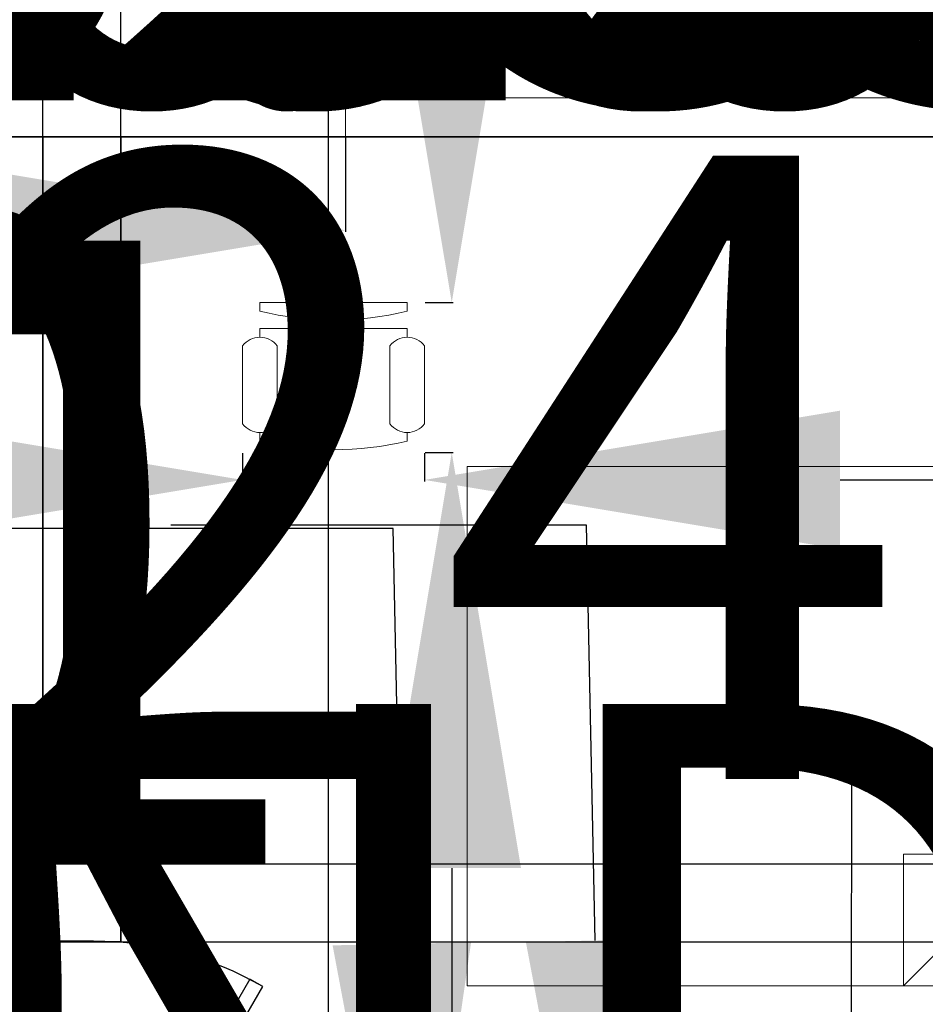
# Model space of a CAD drawing. Units: inches. Extents: x -307 to 2141, y -58 to 895.
# Tile 23 of 28: x 776 to 880, y 582 to 696. Entities that reach past the tile are written whole.
import ezdxf

# ---------------------------------------------------------------- set-up
doc = ezdxf.new("R2010")
doc.units = ezdxf.units.IN
doc.header["$MEASUREMENT"] = 0
for name, color, linetype, lineweight in [('A-ANNO-DIMS', 2, 'Continuous', 18), ('A-DOOR', 3, 'Continuous', 25), ('A-FURN', 8, 'Continuous', 18), ('A-GLAZ', 4, 'Continuous', 18), ('A-WALL', 7, 'Continuous', 35)]:
    doc.layers.add(name, color=color, linetype=linetype, lineweight=lineweight)
doc.styles.get("Standard").update_dxf_attribs({"font": 'arial.ttf'})
doc.dimstyles.get("Standard").update_dxf_attribs({"dimtxt": 72, "dimasz": 48, "dimexe": 0.18, "dimexo": 0.0625, "dimgap": 0.09, "dimtad": 0, "dimtih": 1, "dimtoh": 1, "dimdec": 0, "dimrnd": 48, "dimzin": 0, "dimdsep": 46, "dimlunit": 3, "dimtxsty": 'Standard', "dimcen": 0.09, "dimadec": 0, "dimazin": 0, "dimtfac": 1, "dimtdec": 0, "dimtofl": 0, "dimtmove": 0, "dimatfit": 3, "dimfxl": 1, "dimtolj": 1, "dimtzin": 0, "dimarcsym": 0})

# ---------------------------------------------------------------- blocks, each defined once
blk = doc.blocks.new('*U2')
for p, q in [((0, 0), (0, -6)), ((-40, 0), (-40, -6))]:
    blk.add_line(p, q)
blk.add_lwpolyline([(0, 0), (-34.64, 20), (-35.52, 18.48), (-0.87, -1.52)], close=True)
blk.add_arc((0, 0), 40, 150, 180)
blk = doc.blocks.new('Bed - Queen')
for p, q in [((0, -80.00003), (0, 0)), ((0, 0), (59.99999, 0)), ((59.99999, 0), (59.99999, -80.00003)), ((7.99999, -1.2), (28.79998, -1.2)), ((7.99999, -14.4), (7.99999, -1.2)), ((28.79998, -1.2), (28.79998, -14.4)), ((31.19999, -1.2), (51.99999, -1.2)), ((31.19999, -14.4), (31.19999, -1.2)), ((51.99999, -1.2), (51.99999, -16.4)), ((0, -14.4), (44.8, -14.4)), ((59.99999, -29.6), (44.8, -14.4)), ((44.8, -14.4), (44.8, -29.6)), ((44.8, -16.8), (0, -16.8)), ((51.99999, -16.4), (46.79936, -16.4)), ((44.8, -29.6), (59.99999, -29.6)), ((59.99999, -80.00003), (0, -80.00003))]:
    blk.add_line(p, q)
blk = doc.blocks.new('Chair - Desk')
for p, q in [((-8.5, 0), (-8.5, -1)), ((-8.5, 0), (8.5, 0)), ((8.5, 0), (8.5, -1)), ((-2, -3), (-2, -1.9355)), ((2, -1.9576), (2, -3)), ((-8.5, -3), (-8.5, -4)), ((-8.5, -3), (8.5, -3)), ((8.5, -3), (8.5, -4)), ((-10.5, -5), (-10.5, -14)), ((-6.5, -14), (-6.5, -5)), ((6.5, -5), (6.5, -14)), ((10.5, -14), (10.5, -5)), ((-8.5, -15), (-8.5, -16)), ((8.5, -15), (8.5, -16))]:
    blk.add_line(p, q)
for centre, radius, start, end in [((0, 34.625), 36.625, 256.5803, 283.4197), ((-8.5, -6.5), 2.5, 36.8699, 143.1301), ((8.5, -6.5), 2.5, 36.8699, 143.1301), ((-8.5, -12.5), 2.5, 216.8699, 323.1301), ((8.5, -12.5), 2.5, 216.8699, 323.1301), ((0, 19.625), 36.625, 256.5803, 283.4197)]:
    blk.add_arc(centre, radius, start, end)
blk = doc.blocks.new('WIN-72IN')
blk.add_line((72, 4.5), (0, 4.5))
blk.add_lwpolyline([(72, 0), (0, 0), (0, 9), (72, 9)], close=True)
blk = doc.blocks.new('*D30')
at = {"layer": 'A-ANNO-DIMS', "color": 0, "lineweight": -2, "transparency": 16777216}
for p, q in [((570.74, 532.83), (570.74, 580.83)), ((570.74, 580.83), (618.74, 580.83)), ((565.4, 484.83), (570.92, 484.83)), ((565.4, 448.83), (570.92, 448.83)), ((570.74, 400.83), (570.74, 352.83))]:
    blk.add_line(p, q, dxfattribs=at)
at = {"layer": 'A-ANNO-DIMS', "color": 0, "transparency": 16777216}
for points in [[(562.74, 532.83), (578.74, 532.83), (570.74, 484.83)], [(562.74, 400.83), (578.74, 400.83), (570.74, 448.83)]]:
    blk.add_solid(points, dxfattribs=at)
at = {"layer": 'Defpoints', "color": 0, "transparency": 16777216}
for p in [(565.34, 484.83), (570.74, 484.83), (565.34, 448.83)]:
    blk.add_point(p, dxfattribs=at)
at = {"layer": 'A-ANNO-DIMS', "color": 0, "transparency": 16777216, "insert": (1030.17, 580.83), "char_height": 72, "attachment_point": 5}
blk.add_mtext('\\A1;WINDOW 36 TYP.', dxfattribs=at)
blk = doc.blocks.new('*D32')
at = {"layer": 'A-ANNO-DIMS', "color": 0, "lineweight": -2, "transparency": 16777216}
for p, q in [((813.29, 682.28), (813.29, 671.36)), ((885.29, 682.28), (885.29, 671.36)), ((765.29, 671.54), (717.29, 671.54)), ((933.29, 671.54), (981.29, 671.54))]:
    blk.add_line(p, q, dxfattribs=at)
at = {"layer": 'A-ANNO-DIMS', "color": 0, "transparency": 16777216}
for points in [[(765.29, 679.54), (765.29, 663.54), (813.29, 671.54)], [(933.29, 679.54), (933.29, 663.54), (885.29, 671.54)]]:
    blk.add_solid(points, dxfattribs=at)
at = {"layer": 'Defpoints', "color": 0, "transparency": 16777216}
for p in [(813.29, 682.34), (885.29, 682.34), (885.29, 671.54)]:
    blk.add_point(p, dxfattribs=at)
at = {"layer": 'A-ANNO-DIMS', "color": 0, "transparency": 16777216, "insert": (1392.73, 671.54), "char_height": 72, "attachment_point": 5}
blk.add_mtext('\\A1;WINDOW 72 TYP.', dxfattribs=at)
blk = doc.blocks.new('*D36')
at = {"layer": 'A-ANNO-DIMS', "color": 0, "lineweight": -2, "transparency": 16777216}
for p, q in [((871.71, 562.4), (871.76, 610.4)), ((876.55, 514.4), (871.47, 514.4)), ((876.51, 481.35), (871.44, 481.36)), ((871.56, 433.36), (871.51, 385.36)), ((871.51, 385.36), (823.51, 385.36))]:
    blk.add_line(p, q, dxfattribs=at)
at = {"layer": 'A-ANNO-DIMS', "color": 0, "transparency": 16777216}
for points in [[(863.71, 562.41), (879.71, 562.4), (871.65, 514.4)], [(863.56, 433.37), (879.56, 433.35), (871.62, 481.36)]]:
    blk.add_solid(points, dxfattribs=at)
at = {"layer": 'Defpoints', "color": 0, "transparency": 16777216}
for p in [(876.61, 514.4), (871.62, 481.36), (876.57, 481.35)]:
    blk.add_point(p, dxfattribs=at)
at = {"layer": 'A-ANNO-DIMS', "color": 0, "transparency": 16777216, "insert": (548.95, 385.36), "char_height": 72, "attachment_point": 5}
blk.add_mtext('\\A1;WC 33 TYP.', dxfattribs=at)
blk = doc.blocks.new('*D37')
at = {"layer": 'A-ANNO-DIMS', "color": 0, "lineweight": -2, "transparency": 16777216}
for p, q in [((828.62, 519.41), (780.62, 519.46)), ((876.61, 514.46), (876.62, 519.54)), ((897.61, 514.44), (897.62, 519.51)), ((945.62, 519.28), (993.62, 519.22))]:
    blk.add_line(p, q, dxfattribs=at)
at = {"layer": 'A-ANNO-DIMS', "color": 0, "transparency": 16777216}
for points in [[(828.63, 527.41), (828.61, 511.41), (876.62, 519.36)], [(945.63, 527.28), (945.61, 511.28), (897.62, 519.33)]]:
    blk.add_solid(points, dxfattribs=at)
at = {"layer": 'Defpoints', "color": 0, "transparency": 16777216}
for p in [(876.62, 519.36), (876.61, 514.4), (897.61, 514.38)]:
    blk.add_point(p, dxfattribs=at)
at = {"layer": 'A-ANNO-DIMS', "color": 0, "transparency": 16777216, "insert": (604.68, 519.46), "char_height": 72, "attachment_point": 5}
blk.add_mtext('\\A1;21 TYP.', dxfattribs=at)
blk = doc.blocks.new('*D42')
at = {"layer": 'A-ANNO-DIMS', "color": 0, "lineweight": -2, "transparency": 16777216}
for p, q in [((880.26, 543.86), (928.25, 544.87)), ((822.3, 541.2), (822.27, 542.82)), ((832.3, 541.41), (832.27, 543.03)), ((774.28, 541.63), (726.29, 540.62))]:
    blk.add_line(p, q, dxfattribs=at)
at = {"layer": 'A-ANNO-DIMS', "color": 0, "transparency": 16777216}
for points in [[(880.09, 551.86), (880.43, 535.86), (832.27, 542.85)], [(774.11, 549.63), (774.45, 533.63), (822.27, 542.64)]]:
    blk.add_solid(points, dxfattribs=at)
at = {"layer": 'Defpoints', "color": 0, "transparency": 16777216}
for p in [(832.27, 542.85), (822.3, 541.14), (832.3, 541.35)]:
    blk.add_point(p, dxfattribs=at)
at = {"layer": 'A-ANNO-DIMS', "color": 0, "transparency": 16777216, "insert": (1192.89, 544.87), "char_height": 72, "attachment_point": 5}
blk.add_mtext('\\A1;FAUCET 10', dxfattribs=at)
blk = doc.blocks.new('*D43')
at = {"layer": 'A-ANNO-DIMS', "color": 0, "lineweight": -2, "transparency": 16777216}
for p, q in [((818.79, 637.09), (770.79, 637.09)), ((819.79, 589.1), (818.79, 637.09)), ((822.24, 541.14), (820.62, 541.1)), ((822.38, 534.64), (820.76, 534.61)), ((821.95, 486.62), (822.96, 438.63))]:
    blk.add_line(p, q, dxfattribs=at)
at = {"layer": 'A-ANNO-DIMS', "color": 0, "transparency": 16777216}
for points in [[(827.79, 589.27), (811.8, 588.93), (820.8, 541.11)], [(829.95, 486.79), (813.95, 486.45), (820.94, 534.61)]]:
    blk.add_solid(points, dxfattribs=at)
at = {"layer": 'Defpoints', "color": 0, "transparency": 16777216}
for p in [(820.8, 541.11), (822.3, 541.14), (822.44, 534.64)]:
    blk.add_point(p, dxfattribs=at)
at = {"layer": 'A-ANNO-DIMS', "color": 0, "transparency": 16777216, "insert": (747.39, 637.09), "char_height": 72, "attachment_point": 5}
blk.add_mtext('\\A1;7', dxfattribs=at)
blk = doc.blocks.new('*D44')
at = {"layer": 'A-ANNO-DIMS', "color": 0, "lineweight": -2, "transparency": 16777216}
for p, q in [((839.87, 521.22), (839.95, 517.42)), ((815.33, 520.71), (815.41, 516.91)), ((887.94, 518.61), (935.93, 519.62)), ((767.41, 516.08), (719.42, 515.07))]:
    blk.add_line(p, q, dxfattribs=at)
at = {"layer": 'A-ANNO-DIMS', "color": 0, "transparency": 16777216}
for points in [[(887.77, 526.61), (888.11, 510.61), (839.95, 517.6)], [(767.25, 524.08), (767.58, 508.08), (815.4, 517.09)]]:
    blk.add_solid(points, dxfattribs=at)
at = {"layer": 'Defpoints', "color": 0, "transparency": 16777216}
for p in [(839.87, 521.29), (815.33, 520.77), (839.95, 517.6)]:
    blk.add_point(p, dxfattribs=at)
at = {"layer": 'A-ANNO-DIMS', "color": 0, "transparency": 16777216, "insert": (1151.16, 519.62), "char_height": 72, "attachment_point": 5}
blk.add_mtext('\\A1;BASIN 25', dxfattribs=at)
blk = doc.blocks.new('*D45')
at = {"layer": 'A-ANNO-DIMS', "color": 0, "lineweight": -2, "transparency": 16777216}
for p, q in [((841.11, 637.47), (793.11, 637.47)), ((842.12, 589.48), (841.11, 637.47)), ((839.51, 541.42), (843.31, 541.5)), ((839.93, 521.29), (843.73, 521.37)), ((844.56, 473.37), (845.57, 425.38))]:
    blk.add_line(p, q, dxfattribs=at)
at = {"layer": 'A-ANNO-DIMS', "color": 0, "transparency": 16777216}
for points in [[(850.12, 589.65), (834.12, 589.32), (843.13, 541.49)], [(852.56, 473.54), (836.56, 473.21), (843.55, 521.36)]]:
    blk.add_solid(points, dxfattribs=at)
at = {"layer": 'Defpoints', "color": 0, "transparency": 16777216}
for p in [(843.13, 541.49), (839.45, 541.42), (839.87, 521.29)]:
    blk.add_point(p, dxfattribs=at)
at = {"layer": 'A-ANNO-DIMS', "color": 0, "transparency": 16777216, "insert": (740.96, 637.47), "char_height": 72, "attachment_point": 5}
blk.add_mtext('\\A1;20', dxfattribs=at)
blk = doc.blocks.new('*D46')
at = {"layer": 'A-ANNO-DIMS', "color": 0, "lineweight": -2, "transparency": 16777216}
for p, q in [((801.41, 645.78), (801.41, 642.52)), ((822.41, 645.78), (822.41, 642.52)), ((753.41, 642.7), (705.41, 642.7)), ((870.41, 642.7), (918.41, 642.7))]:
    blk.add_line(p, q, dxfattribs=at)
at = {"layer": 'A-ANNO-DIMS', "color": 0, "transparency": 16777216}
for points in [[(753.41, 650.7), (753.41, 634.7), (801.41, 642.7)], [(870.41, 650.7), (870.41, 634.7), (822.41, 642.7)]]:
    blk.add_solid(points, dxfattribs=at)
at = {"layer": 'Defpoints', "color": 0, "transparency": 16777216}
for p in [(801.41, 645.85), (822.41, 645.85), (822.41, 642.7)]:
    blk.add_point(p, dxfattribs=at)
at = {"layer": 'A-ANNO-DIMS', "color": 0, "transparency": 16777216, "insert": (1282.7, 642.7), "char_height": 72, "attachment_point": 5}
blk.add_mtext('\\A1;DESK CHAIR 21', dxfattribs=at)
blk = doc.blocks.new('*D47')
at = {"layer": 'A-ANNO-DIMS', "color": 0, "lineweight": -2, "transparency": 16777216}
for p, q in [((825.56, 711.18), (825.56, 759.18)), ((825.56, 759.18), (873.56, 759.18)), ((822.48, 663.18), (825.74, 663.18)), ((822.48, 645.85), (825.74, 645.85)), ((825.56, 597.85), (825.56, 549.85))]:
    blk.add_line(p, q, dxfattribs=at)
at = {"layer": 'A-ANNO-DIMS', "color": 0, "transparency": 16777216}
for points in [[(817.56, 711.18), (833.56, 711.18), (825.56, 663.18)], [(817.56, 597.85), (833.56, 597.85), (825.56, 645.85)]]:
    blk.add_solid(points, dxfattribs=at)
at = {"layer": 'Defpoints', "color": 0, "transparency": 16777216}
for p in [(822.41, 663.18), (825.56, 663.18), (822.41, 645.85)]:
    blk.add_point(p, dxfattribs=at)
at = {"layer": 'A-ANNO-DIMS', "color": 0, "transparency": 16777216, "insert": (921.83, 759.18), "char_height": 72, "attachment_point": 5}
blk.add_mtext('\\A1;17', dxfattribs=at)
blk = doc.blocks.new('*D52')
at = {"layer": 'A-ANNO-DIMS', "color": 0, "lineweight": -2, "transparency": 16777216}
for p, q in [((660.21, 554.25), (660.21, 602.25)), ((673.8, 506.25), (660.03, 506.25)), ((673.8, 415.25), (660.03, 415.25)), ((660.21, 367.25), (660.21, 319.25))]:
    blk.add_line(p, q, dxfattribs=at)
at = {"layer": 'A-ANNO-DIMS', "color": 0, "transparency": 16777216}
for points in [[(652.21, 554.25), (668.21, 554.25), (660.21, 506.25)], [(652.21, 367.25), (668.21, 367.25), (660.21, 415.25)]]:
    blk.add_solid(points, dxfattribs=at)
at = {"layer": 'Defpoints', "color": 0, "transparency": 16777216}
for p in [(673.86, 506.25), (660.21, 415.25), (673.86, 415.25)]:
    blk.add_point(p, dxfattribs=at)
at = {"layer": 'A-ANNO-DIMS', "color": 0, "transparency": 16777216, "insert": (660.21, 460.75), "char_height": 72, "attachment_point": 5}
blk.add_mtext('\\A1;DINING SET 91', dxfattribs=at)
blk = doc.blocks.new('*D56')
at = {"layer": 'A-ANNO-DIMS', "color": 0, "lineweight": -2, "transparency": 16777216}
for p, q in [((679.73, 723.21), (679.73, 771.21)), ((679.73, 771.21), (727.73, 771.21)), ((675.74, 675.21), (679.91, 675.21)), ((675.74, 648.21), (679.91, 648.21)), ((679.73, 600.21), (679.73, 552.21))]:
    blk.add_line(p, q, dxfattribs=at)
at = {"layer": 'A-ANNO-DIMS', "color": 0, "transparency": 16777216}
for points in [[(671.73, 723.21), (687.73, 723.21), (679.73, 675.21)], [(671.73, 600.21), (687.73, 600.21), (679.73, 648.21)]]:
    blk.add_solid(points, dxfattribs=at)
at = {"layer": 'Defpoints', "color": 0, "transparency": 16777216}
for p in [(675.68, 675.21), (679.73, 675.21), (675.68, 648.21)]:
    blk.add_point(p, dxfattribs=at)
at = {"layer": 'A-ANNO-DIMS', "color": 0, "transparency": 16777216, "insert": (1006.66, 771.21), "char_height": 72, "attachment_point": 5}
blk.add_mtext('\\A1;ROCKER 27', dxfattribs=at)
blk = doc.blocks.new('*D57')
at = {"layer": 'A-ANNO-DIMS', "color": 0, "lineweight": -2, "transparency": 16777216}
for p, q in [((651.25, 648.15), (651.25, 643.98)), ((675.68, 648.15), (675.68, 643.98)), ((603.25, 644.16), (555.25, 644.16)), ((723.68, 644.16), (771.68, 644.16))]:
    blk.add_line(p, q, dxfattribs=at)
at = {"layer": 'A-ANNO-DIMS', "color": 0, "transparency": 16777216}
for points in [[(603.25, 652.16), (603.25, 636.16), (651.25, 644.16)], [(723.68, 652.16), (723.68, 636.16), (675.68, 644.16)]]:
    blk.add_solid(points, dxfattribs=at)
at = {"layer": 'Defpoints', "color": 0, "transparency": 16777216}
for p in [(651.25, 648.21), (675.68, 648.21), (675.68, 644.16)]:
    blk.add_point(p, dxfattribs=at)
at = {"layer": 'A-ANNO-DIMS', "color": 0, "transparency": 16777216, "insert": (823.81, 644.16), "char_height": 72, "attachment_point": 5}
blk.add_mtext('\\A1;24', dxfattribs=at)
blk = doc.blocks.new('*D62')
at = {"layer": 'A-ANNO-DIMS', "color": 0, "lineweight": -2, "transparency": 16777216}
for p, q in [((556.34, 691.4), (556.34, 722.72)), ((604.34, 722.54), (656.85, 722.54)), ((868.34, 722.54), (815.82, 722.54)), ((916.34, 490.97), (916.34, 722.72))]:
    blk.add_line(p, q, dxfattribs=at)
at = {"layer": 'A-ANNO-DIMS', "color": 0, "transparency": 16777216}
for points in [[(604.34, 730.54), (604.34, 714.54), (556.34, 722.54)], [(868.34, 730.54), (868.34, 714.54), (916.34, 722.54)]]:
    blk.add_solid(points, dxfattribs=at)
at = {"layer": 'Defpoints', "color": 0, "transparency": 16777216}
for p in [(916.34, 722.54), (556.34, 691.34), (916.34, 490.9)]:
    blk.add_point(p, dxfattribs=at)
at = {"layer": 'A-ANNO-DIMS', "color": 0, "transparency": 16777216, "insert": (736.34, 722.54), "char_height": 72, "attachment_point": 5}
blk.add_mtext('\\A1;360', dxfattribs=at)
blk = doc.blocks.new('*D63')
at = {"layer": 'A-ANNO-DIMS', "color": 0, "lineweight": -2, "transparency": 16777216}
for p, q in [((916.4, 691.34), (947.72, 691.34)), ((947.54, 643.34), (947.54, 416.19)), ((947.54, 115.34), (947.54, 342.49)), ((704.68, 67.34), (947.72, 67.34))]:
    blk.add_line(p, q, dxfattribs=at)
at = {"layer": 'A-ANNO-DIMS', "color": 0, "transparency": 16777216}
for points in [[(939.54, 643.34), (955.54, 643.34), (947.54, 691.34)], [(939.54, 115.34), (955.54, 115.34), (947.54, 67.34)]]:
    blk.add_solid(points, dxfattribs=at)
at = {"layer": 'Defpoints', "color": 0, "transparency": 16777216}
for p in [(916.34, 691.34), (704.62, 67.34), (947.54, 67.34)]:
    blk.add_point(p, dxfattribs=at)
at = {"layer": 'A-ANNO-DIMS', "color": 0, "transparency": 16777216, "insert": (947.54, 379.34), "char_height": 72, "attachment_point": 5}
blk.add_mtext('\\A1;624', dxfattribs=at)
blk = doc.blocks.new('*D68')
at = {"layer": 'A-ANNO-DIMS', "color": 0, "lineweight": -2, "transparency": 16777216}
for p, q in [((525.13, 586.34), (525.13, 634.34)), ((525.13, 634.34), (573.13, 634.34)), ((565.27, 538.34), (524.95, 538.34)), ((556.27, 484.83), (524.95, 484.83)), ((525.13, 436.83), (525.13, 388.83))]:
    blk.add_line(p, q, dxfattribs=at)
at = {"layer": 'A-ANNO-DIMS', "color": 0, "transparency": 16777216}
for points in [[(517.13, 586.34), (533.13, 586.34), (525.13, 538.34)], [(517.13, 436.83), (533.13, 436.83), (525.13, 484.83)]]:
    blk.add_solid(points, dxfattribs=at)
at = {"layer": 'Defpoints', "color": 0, "transparency": 16777216}
for p in [(525.13, 538.34), (565.34, 538.34), (556.34, 484.83)]:
    blk.add_point(p, dxfattribs=at)
at = {"layer": 'A-ANNO-DIMS', "color": 0, "transparency": 16777216, "insert": (687.75, 634.34), "char_height": 72, "attachment_point": 5}
blk.add_mtext('\\A1;53.51', dxfattribs=at)
blk = doc.blocks.new('*D75')
at = {"layer": 'A-ANNO-DIMS', "color": 0, "lineweight": -2, "transparency": 16777216}
for p, q in [((565.34, 682.4), (565.34, 722.72)), ((613.34, 722.54), (637.34, 722.54)), ((685.34, 682.4), (685.34, 722.72)), ((685.34, 722.54), (733.34, 722.54))]:
    blk.add_line(p, q, dxfattribs=at)
at = {"layer": 'A-ANNO-DIMS', "color": 0, "transparency": 16777216}
for points in [[(613.34, 730.54), (613.34, 714.54), (565.34, 722.54)], [(637.34, 730.54), (637.34, 714.54), (685.34, 722.54)]]:
    blk.add_solid(points, dxfattribs=at)
at = {"layer": 'Defpoints', "color": 0, "transparency": 16777216}
for p in [(685.34, 722.54), (565.34, 682.34), (685.34, 682.34)]:
    blk.add_point(p, dxfattribs=at)
at = {"layer": 'A-ANNO-DIMS', "color": 0, "transparency": 16777216, "insert": (809.45, 722.54), "char_height": 72, "attachment_point": 5}
blk.add_mtext('\\A1;120', dxfattribs=at)
blk = doc.blocks.new('*D76')
at = {"layer": 'A-ANNO-DIMS', "color": 0, "lineweight": -2, "transparency": 16777216}
for p, q in [((646.34, 722.54), (598.34, 722.54)), ((694.34, 682.4), (694.34, 722.72)), ((778.34, 682.4), (778.34, 722.72)), ((826.34, 722.54), (874.34, 722.54))]:
    blk.add_line(p, q, dxfattribs=at)
at = {"layer": 'A-ANNO-DIMS', "color": 0, "transparency": 16777216}
for points in [[(646.34, 730.54), (646.34, 714.54), (694.34, 722.54)], [(826.34, 730.54), (826.34, 714.54), (778.34, 722.54)]]:
    blk.add_solid(points, dxfattribs=at)
at = {"layer": 'Defpoints', "color": 0, "transparency": 16777216}
for p in [(778.34, 722.54), (694.34, 682.34), (778.34, 682.34)]:
    blk.add_point(p, dxfattribs=at)
at = {"layer": 'A-ANNO-DIMS', "color": 0, "transparency": 16777216, "insert": (925.9, 722.54), "char_height": 72, "attachment_point": 5}
blk.add_mtext('\\A1;84', dxfattribs=at)
blk = doc.blocks.new('*D77')
at = {"layer": 'A-ANNO-DIMS', "color": 0, "lineweight": -2, "transparency": 16777216}
for p, q in [((787.34, 682.4), (787.34, 722.72)), ((835.34, 722.54), (859.34, 722.54)), ((907.34, 682.4), (907.34, 722.72)), ((907.34, 722.54), (955.34, 722.54))]:
    blk.add_line(p, q, dxfattribs=at)
at = {"layer": 'A-ANNO-DIMS', "color": 0, "transparency": 16777216}
for points in [[(835.34, 730.54), (835.34, 714.54), (787.34, 722.54)], [(859.34, 730.54), (859.34, 714.54), (907.34, 722.54)]]:
    blk.add_solid(points, dxfattribs=at)
at = {"layer": 'Defpoints', "color": 0, "transparency": 16777216}
for p in [(907.34, 722.54), (787.34, 682.34), (907.34, 682.34)]:
    blk.add_point(p, dxfattribs=at)
at = {"layer": 'A-ANNO-DIMS', "color": 0, "transparency": 16777216, "insert": (1031.45, 722.54), "char_height": 72, "attachment_point": 5}
blk.add_mtext('\\A1;120', dxfattribs=at)
blk = doc.blocks.new('*D78')
at = {"layer": 'A-ANNO-DIMS', "color": 0, "lineweight": -2, "transparency": 16777216}
for p, q in [((947.53984, 730.340828), (947.53984, 778.340828)), ((778.39834, 682.340828), (947.71984, 682.340828)), ((730.39834, 598.340828), (947.71984, 598.340828)), ((947.53984, 550.340828), (947.53984, 502.340828))]:
    blk.add_line(p, q, dxfattribs=at)
at = {"layer": 'A-ANNO-DIMS', "color": 0, "transparency": 16777216}
for points in [[(939.53984, 730.340828), (955.53984, 730.340828), (947.53984, 682.340828)], [(939.53984, 550.340828), (955.53984, 550.340828), (947.53984, 598.340828)]]:
    blk.add_solid(points, dxfattribs=at)
at = {"layer": 'Defpoints', "color": 0, "transparency": 16777216}
for p in [(778.33584, 682.340828), (947.53984, 682.340828), (730.33584, 598.340828)]:
    blk.add_point(p, dxfattribs=at)
at = {"layer": 'A-ANNO-DIMS', "color": 0, "transparency": 16777216, "insert": (947.53984, 640.340828), "char_height": 72, "attachment_point": 5}
blk.add_mtext('\\A1;84', dxfattribs=at)
blk = doc.blocks.new('*D80')
at = {"layer": 'A-ANNO-DIMS', "color": 0, "lineweight": -2, "transparency": 16777216}
for p, q in [((763.34, 722.54), (715.34, 722.54)), ((811.34, 517.4), (811.34, 722.72)), ((907.34, 541.4), (907.34, 722.72)), ((955.34, 722.54), (1003.34, 722.54))]:
    blk.add_line(p, q, dxfattribs=at)
at = {"layer": 'A-ANNO-DIMS', "color": 0, "transparency": 16777216}
for points in [[(763.34, 730.54), (763.34, 714.54), (811.34, 722.54)], [(955.34, 730.54), (955.34, 714.54), (907.34, 722.54)]]:
    blk.add_solid(points, dxfattribs=at)
at = {"layer": 'Defpoints', "color": 0, "transparency": 16777216}
for p in [(907.34, 722.54), (907.34, 541.34), (811.34, 517.34)]:
    blk.add_point(p, dxfattribs=at)
at = {"layer": 'A-ANNO-DIMS', "color": 0, "transparency": 16777216, "insert": (1054.97, 722.54), "char_height": 72, "attachment_point": 5}
blk.add_mtext('\\A1;96', dxfattribs=at)
blk = doc.blocks.new('*D82')
at = {"layer": 'A-ANNO-DIMS', "color": 0, "lineweight": -2, "transparency": 16777216}
for p, q in [((525.13, 565.34), (525.13, 613.34)), ((525.13, 613.34), (573.13, 613.34)), ((802.27, 517.34), (524.95, 517.34)), ((802.27, 481.34), (524.95, 481.34)), ((525.13, 433.34), (525.13, 385.34))]:
    blk.add_line(p, q, dxfattribs=at)
at = {"layer": 'A-ANNO-DIMS', "color": 0, "transparency": 16777216}
for points in [[(517.13, 565.34), (533.13, 565.34), (525.13, 517.34)], [(517.13, 433.34), (533.13, 433.34), (525.13, 481.34)]]:
    blk.add_solid(points, dxfattribs=at)
at = {"layer": 'Defpoints', "color": 0, "transparency": 16777216}
for p in [(525.13, 517.34), (802.34, 517.34), (802.34, 481.34)]:
    blk.add_point(p, dxfattribs=at)
at = {"layer": 'A-ANNO-DIMS', "color": 0, "transparency": 16777216, "insert": (624.74, 613.34), "char_height": 72, "attachment_point": 5}
blk.add_mtext('\\A1;36', dxfattribs=at)
blk = doc.blocks.new('*D83')
at = {"layer": 'A-ANNO-DIMS', "color": 0, "lineweight": -2, "transparency": 16777216}
for p, q in [((947.54, 538.9), (947.54, 586.9)), ((916.4, 490.9), (947.72, 490.9)), ((907.4, 481.34), (947.72, 481.34)), ((947.54, 433.34), (947.54, 385.34)), ((947.54, 385.34), (899.54, 385.34))]:
    blk.add_line(p, q, dxfattribs=at)
at = {"layer": 'A-ANNO-DIMS', "color": 0, "transparency": 16777216}
for points in [[(939.54, 538.9), (955.54, 538.9), (947.54, 490.9)], [(939.54, 433.34), (955.54, 433.34), (947.54, 481.34)]]:
    blk.add_solid(points, dxfattribs=at)
at = {"layer": 'Defpoints', "color": 0, "transparency": 16777216}
for p in [(916.34, 490.9), (907.34, 481.34), (947.54, 481.34)]:
    blk.add_point(p, dxfattribs=at)
at = {"layer": 'A-ANNO-DIMS', "color": 0, "transparency": 16777216, "insert": (777.97, 385.34), "char_height": 72, "attachment_point": 5}
blk.add_mtext('\\A1;9.563', dxfattribs=at)
blk = doc.blocks.new('*D88')
at = {"layer": 'A-ANNO-DIMS', "color": 0, "lineweight": -2, "transparency": 16777216}
for p, q in [((517.33584, 722.544828), (469.33584, 722.544828)), ((565.33584, 295.403328), (565.33584, 722.724828)), ((754.33584, 271.403328), (754.33584, 722.724828)), ((802.33584, 722.544828), (850.33584, 722.544828))]:
    blk.add_line(p, q, dxfattribs=at)
at = {"layer": 'A-ANNO-DIMS', "color": 0, "transparency": 16777216}
for points in [[(517.33584, 730.544828), (517.33584, 714.544828), (565.33584, 722.544828)], [(802.33584, 730.544828), (802.33584, 714.544828), (754.33584, 722.544828)]]:
    blk.add_solid(points, dxfattribs=at)
at = {"layer": 'Defpoints', "color": 0, "transparency": 16777216}
for p in [(754.33584, 722.544828), (565.33584, 295.340828), (754.33584, 271.340828)]:
    blk.add_point(p, dxfattribs=at)
at = {"layer": 'A-ANNO-DIMS', "color": 0, "transparency": 16777216, "insert": (659.83584, 722.544828), "char_height": 72, "attachment_point": 5}
blk.add_mtext('\\A1;189', dxfattribs=at)
blk = doc.blocks.new('*D94')
at = {"layer": 'A-ANNO-DIMS', "color": 0, "lineweight": -2, "transparency": 16777216}
for p, q in [((517.34, 722.54), (469.34, 722.54)), ((565.34, 529.4), (565.34, 722.72)), ((629.84, 529.4), (629.84, 722.72)), ((677.84, 722.54), (725.84, 722.54))]:
    blk.add_line(p, q, dxfattribs=at)
at = {"layer": 'A-ANNO-DIMS', "color": 0, "transparency": 16777216}
for points in [[(517.34, 730.54), (517.34, 714.54), (565.34, 722.54)], [(677.84, 730.54), (677.84, 714.54), (629.84, 722.54)]]:
    blk.add_solid(points, dxfattribs=at)
at = {"layer": 'Defpoints', "color": 0, "transparency": 16777216}
for p in [(629.84, 722.54), (565.34, 529.34), (629.84, 529.34)]:
    blk.add_point(p, dxfattribs=at)
at = {"layer": 'A-ANNO-DIMS', "color": 0, "transparency": 16777216, "insert": (819.9, 722.54), "char_height": 72, "attachment_point": 5}
blk.add_mtext('\\A1;64.5', dxfattribs=at)
blk = doc.blocks.new('*D95')
at = {"layer": 'A-ANNO-DIMS', "color": 0, "lineweight": -2, "transparency": 16777216}
for p, q in [((947.54, 577.34), (947.54, 625.34)), ((947.54, 625.34), (995.54, 625.34)), ((629.9, 529.34), (947.72, 529.34)), ((629.9, 502.66), (947.72, 502.66)), ((947.54, 454.66), (947.54, 406.66))]:
    blk.add_line(p, q, dxfattribs=at)
at = {"layer": 'A-ANNO-DIMS', "color": 0, "transparency": 16777216}
for points in [[(939.54, 577.34), (955.54, 577.34), (947.54, 529.34)], [(939.54, 454.66), (955.54, 454.66), (947.54, 502.66)]]:
    blk.add_solid(points, dxfattribs=at)
at = {"layer": 'Defpoints', "color": 0, "transparency": 16777216}
for p in [(629.84, 529.34), (947.54, 529.34), (629.84, 502.66)]:
    blk.add_point(p, dxfattribs=at)
at = {"layer": 'A-ANNO-DIMS', "color": 0, "transparency": 16777216, "insert": (1117.8, 625.34), "char_height": 72, "attachment_point": 5}
blk.add_mtext('\\A1;26.68', dxfattribs=at)
blk = doc.blocks.new('*D96')
at = {"layer": 'A-ANNO-DIMS', "color": 0, "lineweight": -2, "transparency": 16777216}
for p, q in [((646.34, 722.54), (598.34, 722.54)), ((694.34, 598.4), (694.34, 722.72)), ((730.34, 598.4), (730.34, 722.72)), ((778.34, 722.54), (826.34, 722.54))]:
    blk.add_line(p, q, dxfattribs=at)
at = {"layer": 'A-ANNO-DIMS', "color": 0, "transparency": 16777216}
for points in [[(646.34, 730.54), (646.34, 714.54), (694.34, 722.54)], [(778.34, 730.54), (778.34, 714.54), (730.34, 722.54)]]:
    blk.add_solid(points, dxfattribs=at)
at = {"layer": 'Defpoints', "color": 0, "transparency": 16777216}
for p in [(730.34, 722.54), (694.34, 598.34), (730.34, 598.34)]:
    blk.add_point(p, dxfattribs=at)
at = {"layer": 'A-ANNO-DIMS', "color": 0, "transparency": 16777216, "insert": (877.95, 722.54), "char_height": 72, "attachment_point": 5}
blk.add_mtext('\\A1;36', dxfattribs=at)
blk = doc.blocks.new('*D97')
at = {"layer": 'A-ANNO-DIMS', "color": 0, "lineweight": -2, "transparency": 16777216}
for p, q in [((947.54, 637.34), (947.54, 685.34)), ((947.54, 685.34), (995.54, 685.34)), ((685.4, 589.34), (947.72, 589.34)), ((685.4, 538.34), (947.72, 538.34)), ((947.54, 490.34), (947.54, 442.34))]:
    blk.add_line(p, q, dxfattribs=at)
at = {"layer": 'A-ANNO-DIMS', "color": 0, "transparency": 16777216}
for points in [[(939.54, 637.34), (955.54, 637.34), (947.54, 589.34)], [(939.54, 490.34), (955.54, 490.34), (947.54, 538.34)]]:
    blk.add_solid(points, dxfattribs=at)
at = {"layer": 'Defpoints', "color": 0, "transparency": 16777216}
for p in [(685.34, 589.34), (947.54, 589.34), (685.34, 538.34)]:
    blk.add_point(p, dxfattribs=at)
at = {"layer": 'A-ANNO-DIMS', "color": 0, "transparency": 16777216, "insert": (1040.25, 685.34), "char_height": 72, "attachment_point": 5}
blk.add_mtext('\\A1;51', dxfattribs=at)
blk = doc.blocks.new('*D98')
at = {"layer": 'A-ANNO-DIMS', "color": 0, "lineweight": -2, "transparency": 16777216}
for p, q in [((525.13, 637.34), (525.13, 685.34)), ((525.13, 685.34), (573.13, 685.34)), ((787.27, 589.34), (524.95, 589.34)), ((787.27, 550.34), (524.95, 550.34)), ((525.13, 502.34), (525.13, 454.34))]:
    blk.add_line(p, q, dxfattribs=at)
at = {"layer": 'A-ANNO-DIMS', "color": 0, "transparency": 16777216}
for points in [[(517.13, 637.34), (533.13, 637.34), (525.13, 589.34)], [(517.13, 502.34), (533.13, 502.34), (525.13, 550.34)]]:
    blk.add_solid(points, dxfattribs=at)
at = {"layer": 'Defpoints', "color": 0, "transparency": 16777216}
for p in [(525.13, 589.34), (787.34, 589.34), (787.34, 550.34)]:
    blk.add_point(p, dxfattribs=at)
at = {"layer": 'A-ANNO-DIMS', "color": 0, "transparency": 16777216, "insert": (624.84, 685.34), "char_height": 72, "attachment_point": 5}
blk.add_mtext('\\A1;39', dxfattribs=at)
blk = doc.blocks.new('*D101')
at = {"layer": 'A-ANNO-DIMS', "color": 0, "lineweight": -2, "transparency": 16777216}
for p, q in [((508.34, 722.54), (460.34, 722.54)), ((556.34, 691.4), (556.34, 722.72)), ((589.36, 691.4), (589.36, 722.72)), ((637.36, 722.54), (685.36, 722.54))]:
    blk.add_line(p, q, dxfattribs=at)
at = {"layer": 'A-ANNO-DIMS', "color": 0, "transparency": 16777216}
for points in [[(508.34, 730.54), (508.34, 714.54), (556.34, 722.54)], [(637.36, 730.54), (637.36, 714.54), (589.36, 722.54)]]:
    blk.add_solid(points, dxfattribs=at)
at = {"layer": 'Defpoints', "color": 0, "transparency": 16777216}
for p in [(589.36, 722.54), (556.34, 691.34), (589.36, 691.34)]:
    blk.add_point(p, dxfattribs=at)
at = {"layer": 'A-ANNO-DIMS', "color": 0, "transparency": 16777216, "insert": (806.54, 722.54), "char_height": 72, "attachment_point": 5}
blk.add_mtext('\\A1;33.02', dxfattribs=at)
blk = doc.blocks.new('*D102')
at = {"layer": 'A-ANNO-DIMS', "color": 0, "lineweight": -2, "transparency": 16777216}
for p, q in [((837.29, 722.54), (789.29, 722.54)), ((885.29, 691.4), (885.29, 722.72)), ((916.34, 691.4), (916.34, 722.72)), ((964.34, 722.54), (1012.34, 722.54))]:
    blk.add_line(p, q, dxfattribs=at)
at = {"layer": 'A-ANNO-DIMS', "color": 0, "transparency": 16777216}
for points in [[(837.29, 730.54), (837.29, 714.54), (885.29, 722.54)], [(964.34, 730.54), (964.34, 714.54), (916.34, 722.54)]]:
    blk.add_solid(points, dxfattribs=at)
at = {"layer": 'Defpoints', "color": 0, "transparency": 16777216}
for p in [(916.34, 722.54), (885.29, 691.34), (916.34, 691.34)]:
    blk.add_point(p, dxfattribs=at)
at = {"layer": 'A-ANNO-DIMS', "color": 0, "transparency": 16777216, "insert": (1133.74, 722.54), "char_height": 72, "attachment_point": 5}
blk.add_mtext('\\A1;31.04', dxfattribs=at)
blk = doc.blocks.new('*D103')
at = {"layer": 'A-ANNO-DIMS', "color": 0, "lineweight": -2, "transparency": 16777216}
for p, q in [((637.34, 722.54), (589.34, 722.54)), ((685.34, 682.4), (685.34, 722.72)), ((694.34, 682.4), (694.34, 722.72)), ((742.34, 722.54), (790.34, 722.54))]:
    blk.add_line(p, q, dxfattribs=at)
at = {"layer": 'A-ANNO-DIMS', "color": 0, "transparency": 16777216}
for points in [[(637.34, 730.54), (637.34, 714.54), (685.34, 722.54)], [(742.34, 730.54), (742.34, 714.54), (694.34, 722.54)]]:
    blk.add_solid(points, dxfattribs=at)
at = {"layer": 'Defpoints', "color": 0, "transparency": 16777216}
for p in [(694.34, 722.54), (685.34, 682.34), (694.34, 682.34)]:
    blk.add_point(p, dxfattribs=at)
at = {"layer": 'A-ANNO-DIMS', "color": 0, "transparency": 16777216, "insert": (814.1, 722.54), "char_height": 72, "attachment_point": 5}
blk.add_mtext('\\A1;9', dxfattribs=at)
blk = doc.blocks.new('*D107')
at = {"layer": 'A-ANNO-DIMS', "color": 0, "lineweight": -2, "transparency": 16777216}
for p, q in [((517.34, 722.54), (469.34, 722.54)), ((565.34, 409.4), (565.34, 722.72)), ((589.34, 409.4), (589.34, 722.72)), ((637.34, 722.54), (685.34, 722.54))]:
    blk.add_line(p, q, dxfattribs=at)
at = {"layer": 'A-ANNO-DIMS', "color": 0, "transparency": 16777216}
for points in [[(517.34, 730.54), (517.34, 714.54), (565.34, 722.54)], [(637.34, 730.54), (637.34, 714.54), (589.34, 722.54)]]:
    blk.add_solid(points, dxfattribs=at)
at = {"layer": 'Defpoints', "color": 0, "transparency": 16777216}
for p in [(589.34, 722.54), (565.34, 409.34), (589.34, 409.34)]:
    blk.add_point(p, dxfattribs=at)
at = {"layer": 'A-ANNO-DIMS', "color": 0, "transparency": 16777216, "insert": (835.49, 722.54), "char_height": 72, "attachment_point": 5}
blk.add_mtext('\\A1;24.003', dxfattribs=at)
blk = doc.blocks.new('*D108')
at = {"layer": 'A-ANNO-DIMS', "color": 0, "lineweight": -2, "transparency": 16777216}
for p, q in [((947.54, 550.66), (947.54, 598.66)), ((589.4, 502.66), (947.72, 502.66)), ((589.4, 409.34), (947.72, 409.34)), ((947.54, 361.34), (947.54, 313.34))]:
    blk.add_line(p, q, dxfattribs=at)
at = {"layer": 'A-ANNO-DIMS', "color": 0, "transparency": 16777216}
for points in [[(939.54, 550.66), (955.54, 550.66), (947.54, 502.66)], [(939.54, 361.34), (955.54, 361.34), (947.54, 409.34)]]:
    blk.add_solid(points, dxfattribs=at)
at = {"layer": 'Defpoints', "color": 0, "transparency": 16777216}
for p in [(589.34, 502.66), (947.54, 502.66), (589.34, 409.34)]:
    blk.add_point(p, dxfattribs=at)
at = {"layer": 'A-ANNO-DIMS', "color": 0, "transparency": 16777216, "insert": (947.54, 456), "char_height": 72, "attachment_point": 5}
blk.add_mtext('\\A1;93.32', dxfattribs=at)

msp = doc.modelspace()

# ---------------------------------------------------------------- linework, layer by layer
at = {"layer": 'A-WALL'}
for p, q in [((916.3358, 691.3408), (556.3358, 691.3408)), ((907.3358, 682.3408), (565.3358, 682.3408)), ((778.3358, 589.3408), (778.3358, 682.3408)), ((787.3358, 589.3408), (787.3358, 682.3408)), ((787.3358, 598.3408), (730.3358, 598.3408)), ((787.3358, 589.3408), (730.3358, 589.3408))]:
    msp.add_line(p, q, dxfattribs=at)

# ---------------------------------------------------------------- block references
at = {"layer": 'A-DOOR', "xscale": 0.9766664716736615, "yscale": 0.9766664716736615, "zscale": 0.9766664716736615, "rotation": 270}
msp.add_blockref('*U2', (784.1958, 550.3408), dxfattribs=at)
at = {"layer": 'A-FURN'}
msp.add_blockref('Chair - Desk', (811.9132, 663.1793), dxfattribs=at)
at = {"layer": 'A-FURN', "rotation": 270}
msp.add_blockref('Bed - Queen', (907.3358, 644.2648), dxfattribs=at)
at = {"layer": 'A-GLAZ'}
msp.add_blockref('WIN-72IN', (813.293, 682.341), dxfattribs=at)

# ---------------------------------------------------------------- dimensions: what is measured, and where the dimension line sits
at = {"layer": 'A-ANNO-DIMS'}
for base, p1, p2, angle, text, picture, middle in [((679.7317, 675.211), (675.6817, 648.211), (675.6817, 675.211), 90, 'ROCKER <>', '*D56', (1006.6621, 771.211)), ((570.7358, 484.8333), (565.3358, 448.8333), (565.3358, 484.8333), 90, 'WINDOW <> TYP.', '*D30', (1030.1737, 580.8333)), ((832.2692, 542.8502), (822.3029, 541.1403), (832.3007, 541.3505), 1.204628, 'FAUCET <>', '*D42', (1192.8864, 544.8684)), ((660.2083, 415.2485), (673.8583, 506.2485), (673.8583, 415.2485), 270, 'DINING SET <>', '*D52', (660.2083, 460.7485)), ((876.6162, 519.3557), (897.6106, 514.3753), (876.6106, 514.3988), 179.935892, '<> TYP.', '*D37', (604.6763, 519.4631)), ((839.9481, 517.6035), (815.3253, 520.7692), (839.8707, 521.2853), 1.204628, 'BASIN <>', '*D44', (1151.1574, 519.6217)), ((871.6167, 481.3581), (876.6106, 514.3988), (876.5736, 481.3526), 269.935892, 'WC <> TYP.', '*D36', (548.95, 385.3582))]:
    dim = msp.add_linear_dim(base=base, p1=p1, p2=p2, angle=angle, text=text, dimstyle='Standard', override={"dimdec": 0, "dimlfac": 1, "dimrnd": 0, "dimzin": 0, "dimdsep": 46, "dimlunit": 2}, dxfattribs=at)
    dim.commit()
    dim.dimension.update_dxf_attribs({"geometry": picture, "text_midpoint": middle})
for base, p1, p2, text, picture, middle in [((885.2934, 671.5408), (813.2934, 682.3408), (885.2934, 682.3408), 'WINDOW <> TYP.', '*D32', (1392.7312, 671.5408)), ((822.4132, 642.696), (801.4132, 645.846), (822.4132, 645.846), 'DESK CHAIR <>', '*D46', (1282.7024, 642.696))]:
    dim = msp.add_linear_dim(base=base, p1=p1, p2=p2, text=text, dimstyle='Standard', override={"dimdec": 0, "dimlfac": 1, "dimrnd": 0, "dimzin": 0, "dimdsep": 46, "dimlunit": 2}, dxfattribs=at)
    dim.commit()
    dim.dimension.update_dxf_attribs({"geometry": picture, "text_midpoint": middle})
for base, p1, p2, angle, override, picture, middle in [((825.5632, 663.1793), (822.4132, 645.846), (822.4132, 663.1793), 90, {"dimdec": 0, "dimlfac": 1, "dimrnd": 0, "dimzin": 0, "dimdsep": 46, "dimlunit": 2}, '*D47', (921.8333, 759.1793)), ((947.5398, 682.3408), (730.3358, 598.3408), (778.3358, 682.3408), 90, {"dimdec": 0, "dimlfac": 1, "dimrnd": 0, "dimzin": 0, "dimdsep": 46, "dimlunit": 2}, '*D78', (947.5398, 640.3408)), ((525.1318, 589.3408), (787.3358, 550.3408), (787.3358, 589.3408), 90, {"dimdec": 0, "dimlfac": 1, "dimrnd": 0, "dimzin": 0, "dimdsep": 46, "dimlunit": 2}, '*D98', (624.8398, 685.3408)), ((947.5398, 589.3408), (685.3358, 538.3408), (685.3358, 589.3408), 90, {"dimdec": 0, "dimlfac": 1, "dimrnd": 0, "dimzin": 0, "dimdsep": 46, "dimlunit": 2}, '*D97', (1040.2492, 685.3408)), ((947.5398, 67.3408), (916.3358, 691.3408), (704.6211, 67.3408), 90, {"dimdec": 0, "dimlfac": 1, "dimrnd": 0, "dimzin": 0, "dimdsep": 46, "dimlunit": 2}, '*D63', (947.5398, 379.3408)), ((843.1292, 541.4949), (839.8707, 521.2853), (839.4474, 541.4175), 91.204628, {"dimdec": 0, "dimlfac": 1, "dimrnd": 0, "dimzin": 0, "dimdsep": 46, "dimlunit": 2}, '*D45', (740.961, 637.4737)), ((820.8033, 541.1087), (822.4396, 534.6416), (822.3029, 541.1403), 91.204628, {"dimdec": 0, "dimlfac": 1, "dimrnd": 0, "dimzin": 0, "dimdsep": 46, "dimlunit": 2}, '*D43', (747.3908, 637.0875)), ((525.1318, 538.3408), (556.3358, 484.8333), (565.3358, 538.3408), 90, {"dimdec": 2, "dimlfac": 1, "dimrnd": 0, "dimzin": 0, "dimdsep": 46, "dimlunit": 2}, '*D68', (687.7539, 634.3408)), ((947.5398, 529.3408), (629.8358, 502.6632), (629.8358, 529.3408), 90, {"dimdec": 2, "dimlfac": 1, "dimrnd": 0, "dimzin": 0, "dimdsep": 46, "dimlunit": 2}, '*D95', (1117.799, 625.3408)), ((525.1318, 517.3408), (802.3358, 481.3408), (802.3358, 517.3408), 90, {"dimdec": 0, "dimlfac": 1, "dimrnd": 0, "dimzin": 0, "dimdsep": 46, "dimlunit": 2}, '*D82', (624.7416, 613.3408)), ((947.5398, 502.6632), (589.339, 409.3408), (589.339, 502.6632), 90, {"dimdec": 2, "dimlfac": 1, "dimrnd": 0, "dimzin": 0, "dimdsep": 46, "dimlunit": 2}, '*D108', (947.5398, 456.002)), ((947.5398, 481.3408), (916.3358, 490.9034), (907.3358, 481.3408), 90, {"dimdec": 3, "dimlfac": 1, "dimrnd": 0, "dimzin": 0, "dimdsep": 46, "dimlunit": 2}, '*D83', (777.9683, 385.3408))]:
    dim = msp.add_linear_dim(base=base, p1=p1, p2=p2, angle=angle, dimstyle='Standard', override=override, dxfattribs=at)
    dim.commit()
    dim.dimension.update_dxf_attribs({"geometry": picture, "text_midpoint": middle})
for base, p1, p2, override, picture, middle in [((589.3579, 722.5448), (556.3358, 691.3408), (589.3579, 691.3408), {"dimdec": 2, "dimlfac": 1, "dimrnd": 0, "dimzin": 0, "dimdsep": 46, "dimlunit": 2}, '*D101', (806.5366, 722.5448)), ((754.3358, 722.5448), (565.3358, 295.3408), (754.3358, 271.3408), {"dimdec": 0, "dimlfac": 1, "dimrnd": 0, "dimzin": 0, "dimdsep": 46, "dimlunit": 2}, '*D88', (659.8358, 722.5448)), ((629.8358, 722.5448), (565.3358, 529.3408), (629.8358, 529.3408), {"dimdec": 1, "dimlfac": 1, "dimrnd": 0, "dimzin": 0, "dimdsep": 46, "dimlunit": 2}, '*D94', (819.904, 722.5448)), ((589.339, 722.5448), (565.3358, 409.3408), (589.339, 409.3408), {"dimdec": 3, "dimlfac": 1, "dimrnd": 0, "dimzin": 0, "dimdsep": 46, "dimlunit": 2}, '*D107', (835.4945, 722.5448)), ((916.3358, 722.5448), (556.3358, 691.3408), (916.3358, 490.9034), {"dimdec": 0, "dimlfac": 1, "dimrnd": 0, "dimzin": 0, "dimdsep": 46, "dimlunit": 2}, '*D62', (736.3358, 722.5448)), ((685.3358, 722.5448), (565.3358, 682.3408), (685.3358, 682.3408), {"dimdec": 0, "dimlfac": 1, "dimrnd": 0, "dimzin": 0, "dimdsep": 46, "dimlunit": 2}, '*D75', (809.4531, 722.5448)), ((694.3358, 722.5448), (685.3358, 682.3408), (694.3358, 682.3408), {"dimdec": 0, "dimlfac": 1, "dimrnd": 0, "dimzin": 0, "dimdsep": 46, "dimlunit": 2}, '*D103', (814.0984, 722.5448)), ((778.3358, 722.5448), (694.3358, 682.3408), (778.3358, 682.3408), {"dimdec": 0, "dimlfac": 1, "dimrnd": 0, "dimzin": 0, "dimdsep": 46, "dimlunit": 2}, '*D76', (925.8965, 722.5448)), ((730.3358, 722.5448), (694.3358, 598.3408), (730.3358, 598.3408), {"dimdec": 0, "dimlfac": 1, "dimrnd": 0, "dimzin": 0, "dimdsep": 46, "dimlunit": 2}, '*D96', (877.9456, 722.5448)), ((907.3358, 722.5448), (811.3358, 517.3408), (907.3358, 541.3408), {"dimdec": 0, "dimlfac": 1, "dimrnd": 0, "dimzin": 0, "dimdsep": 46, "dimlunit": 2}, '*D80', (1054.9702, 722.5448)), ((907.3358, 722.5448), (787.3358, 682.3408), (907.3358, 682.3408), {"dimdec": 0, "dimlfac": 1, "dimrnd": 0, "dimzin": 0, "dimdsep": 46, "dimlunit": 2}, '*D77', (1031.4531, 722.5448)), ((916.3358, 722.5448), (885.2934, 691.3408), (916.3358, 691.3408), {"dimdec": 2, "dimlfac": 1, "dimrnd": 0, "dimzin": 0, "dimdsep": 46, "dimlunit": 2}, '*D102', (1133.7355, 722.5448)), ((675.6817, 644.161), (651.2466, 648.211), (675.6817, 648.211), {"dimdec": 0, "dimlfac": 1, "dimrnd": 0, "dimzin": 0, "dimdsep": 46, "dimlunit": 2}, '*D57', (823.8072, 644.161))]:
    dim = msp.add_linear_dim(base=base, p1=p1, p2=p2, dimstyle='Standard', override=override, dxfattribs=at)
    dim.commit()
    dim.dimension.update_dxf_attribs({"geometry": picture, "text_midpoint": middle})

doc.saveas('drawing.dxf')
